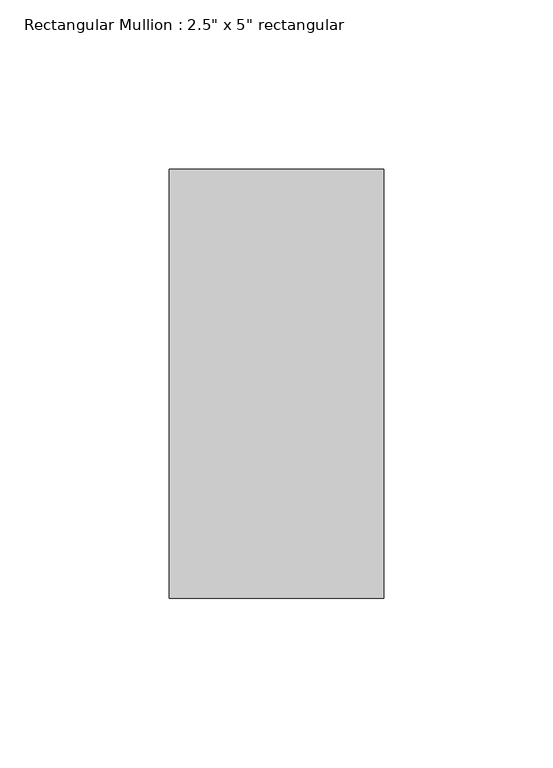
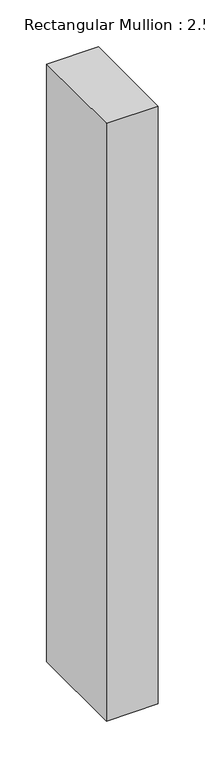
"""IFC4 building model written with IfcOpenShell, lengths in millimetres: member geometry."""

from ifc_helpers import new_model, si_unit, frame, origin, place, context, project, spatial, polyline, outline, extrude, source, transform, mapped, element, save


def member_613aa8fe(model_context):
    return source(origin(), model_context, "Body", "SweptSolid", [
        extrude(outline(polyline([(0.0, 63.5), (0.0, -63.5), (-63.5, -63.5), (-63.5, 63.5), (0.0, 63.5)])), frame((0.0, 0.0, -776.6032277), z_axis=(0.0, 0.0, 1.0), x_axis=(1.0, 0.0, 0.0)), (0.0, 0.0, 1.0), 776.6032277),
    ])


if __name__ == "__main__":
    model = new_model("IFC4")
    model_context = context("Model", 3, world=origin())
    ifc_project = project(units=[si_unit("LENGTHUNIT", "METRE", prefix="MILLI")], contexts=[model_context])
    site = spatial("IfcSite", under=ifc_project)
    building = spatial("IfcBuilding", under=site)
    placement = place(None, origin())
    member_shape = member_613aa8fe(model_context)
    element("IfcMember", 1, ObjectType="Rectangular Mullion : 2.5\" x 5\" rectangular", at=placement, inside=building, context=model_context, shape_type="MappedRepresentation", body=[
        mapped(member_shape, transform((0.0, 0.0, 0.0), x_axis=(1.0, 0.0, 0.0), y_axis=(0.0, 1.0, 0.0), z_axis=(0.0, 0.0, 1.0))),
    ])
    save(model, "model.ifc")

# Revit data of these elements
# Type "Rectangular Mullion : 2.5\" x 5\" rectangular"
#   built-in parameter 1007304 = 0.416667 (stored number, unit not read)
#   built-in parameter 1007301 = 0.104167 (stored number, unit not read)
#   built-in parameter 1007300 = 0.104167 (stored number, unit not read)
# Element 1 (IfcMember, "Rectangular Mullion : 2.5\" x 5\" rectangular")
#   Materials on its faces: "Aluminum"
# Materials
#   "Aluminum": class "Metal", colour RGB 247 247 247, transparency 0, Description = "Aluminum 6061", Cost = 0
